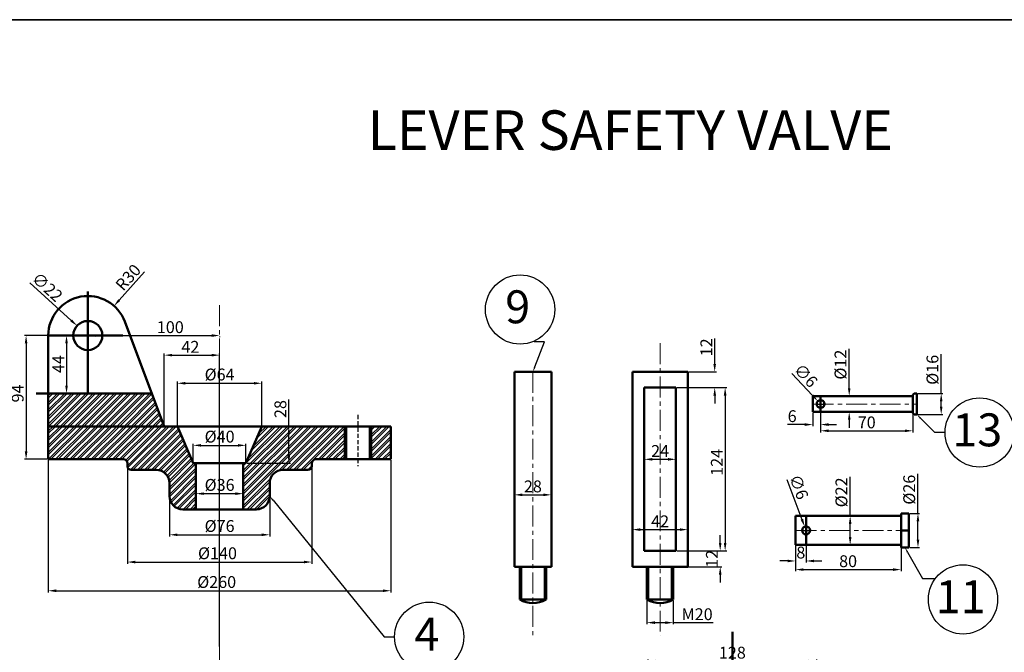
# Model space of a CAD drawing. Units: millimetres. Extents: x -282 to 2335, y -1129 to 664.
# Tile 6 of 8: x 594 to 1341, y 183 to 664. Entities that reach past the tile are written whole.
import ezdxf
from ezdxf import colors
from ezdxf.entities.mleader import LeaderData, LeaderLine
from ezdxf.math import Vec2, Vec3

# ---------------------------------------------------------------- set-up
doc = ezdxf.new("R2010")
doc.units = ezdxf.units.MM
doc.header["$LTSCALE"] = 0.5
doc.linetypes.add('CENTER', pattern=[50.8, 31.75, -6.35, 6.35, -6.35])
doc.linetypes.add('HIDDEN', pattern=[9.525, 6.35, -3.175])
for name, color, linetype, lineweight in [('M-CNTR', 1, 'CENTER', 18), ('M-DIMS', 2, 'Continuous', 25), ('M-HATC', 8, 'Continuous', 18), ('M-HIDN', 4, 'HIDDEN', 25), ('M-OUTL', 7, 'Continuous', 50), ('M-TEXT', 3, 'Continuous', 25), ('M-TTLB', 7, 'Continuous', 35)]:
    doc.layers.add(name, color=color, linetype=linetype, lineweight=lineweight)
doc.styles.get("Standard").update_dxf_attribs({"font": 'arial.ttf'})
doc.dimstyles.new('ISO-25', dxfattribs={"dimtxt": 9, "dimasz": 6, "dimexe": 1.25, "dimexo": 0.625, "dimtad": 1, "dimtxsty": 'Standard', "dimcen": 2.5, "dimadec": 0, "dimazin": 0, "dimtfac": 1, "dimtofl": 0, "dimtmove": 0, "dimatfit": 3, "dimfxl": 1, "dimarcsym": 0})

# ---------------------------------------------------------------- blocks, each defined once
blk = doc.blocks.new('*D30')
at = {"layer": 'Defpoints', "color": 0, "transparency": 16777216}
for p in [(645.29, 423.91), (629.15, 379.91), (645.29, 379.91)]:
    blk.add_point(p, dxfattribs=at)
at = {"layer": 'M-DIMS', "color": 0, "lineweight": -2, "transparency": 16777216}
for p, q in [((644.66, 423.91), (627.9, 423.91)), ((629.15, 417.91), (629.15, 385.91)), ((644.66, 379.91), (627.9, 379.91))]:
    blk.add_line(p, q, dxfattribs=at)
at = {"layer": 'M-DIMS', "color": 0, "transparency": 16777216}
for points in [[(628.15, 417.91), (630.15, 417.91), (629.15, 423.91)], [(628.15, 385.91), (630.15, 385.91), (629.15, 379.91)]]:
    blk.add_solid(points, dxfattribs=at)
at = {"layer": 'M-DIMS', "color": 0, "transparency": 16777216, "insert": (624.02, 402.22), "char_height": 9, "attachment_point": 5, "rotation": 90}
blk.add_mtext('44', dxfattribs=at)
blk = doc.blocks.new('*D31')
at = {"layer": 'Defpoints', "color": 0, "transparency": 16777216}
for p in [(645.29, 423.91), (598.46, 329.91), (615.29, 329.91)]:
    blk.add_point(p, dxfattribs=at)
at = {"layer": 'M-DIMS', "color": 0, "lineweight": -2, "transparency": 16777216}
for p, q in [((644.66, 423.91), (597.21, 423.91)), ((598.46, 417.91), (598.46, 335.91)), ((614.66, 329.91), (597.21, 329.91))]:
    blk.add_line(p, q, dxfattribs=at)
at = {"layer": 'M-DIMS', "color": 0, "transparency": 16777216}
for points in [[(597.46, 417.91), (599.46, 417.91), (598.46, 423.91)], [(597.46, 335.91), (599.46, 335.91), (598.46, 329.91)]]:
    blk.add_solid(points, dxfattribs=at)
at = {"layer": 'M-DIMS', "color": 0, "transparency": 16777216, "insert": (593.24, 379.91), "char_height": 9, "attachment_point": 5, "rotation": 90}
blk.add_mtext('94', dxfattribs=at)
blk = doc.blocks.new('*D32')
at = {"layer": 'Defpoints', "color": 0, "transparency": 16777216}
for p in [(645.29, 423.91), (745.29, 423.91), (745.29, 423.88)]:
    blk.add_point(p, dxfattribs=at)
at = {"layer": 'M-DIMS', "color": 0, "lineweight": -2, "transparency": 16777216}
for p, q in [((645.29, 423.29), (645.29, 422.63)), ((651.29, 423.88), (739.29, 423.88)), ((745.29, 423.29), (745.29, 422.63))]:
    blk.add_line(p, q, dxfattribs=at)
at = {"layer": 'M-DIMS', "color": 0, "transparency": 16777216}
for points in [[(651.29, 424.88), (651.29, 422.88), (645.29, 423.88)], [(739.29, 424.88), (739.29, 422.88), (745.29, 423.88)]]:
    blk.add_solid(points, dxfattribs=at)
at = {"layer": 'M-DIMS', "color": 0, "transparency": 16777216, "insert": (707.89, 429.1), "char_height": 9, "attachment_point": 5}
blk.add_mtext('100', dxfattribs=at)
blk = doc.blocks.new('*D33')
at = {"layer": 'Defpoints', "color": 0, "transparency": 16777216}
for p in [(745.29, 409), (703.29, 354.91), (745.29, 187.04)]:
    blk.add_point(p, dxfattribs=at)
at = {"layer": 'M-DIMS', "color": 0, "lineweight": -2, "transparency": 16777216}
for p, q in [((703.29, 355.54), (703.29, 410.25)), ((709.29, 409), (739.29, 409)), ((745.29, 187.66), (745.29, 410.25))]:
    blk.add_line(p, q, dxfattribs=at)
at = {"layer": 'M-DIMS', "color": 0, "transparency": 16777216}
for points in [[(709.29, 410), (709.29, 408), (703.29, 409)], [(739.29, 410), (739.29, 408), (745.29, 409)]]:
    blk.add_solid(points, dxfattribs=at)
at = {"layer": 'M-DIMS', "color": 0, "transparency": 16777216, "insert": (723.11, 414.14), "char_height": 9, "attachment_point": 5}
blk.add_mtext('42', dxfattribs=at)
blk = doc.blocks.new('*D34')
at = {"layer": 'Defpoints', "color": 0, "transparency": 16777216}
for p in [(777.29, 387.65), (713.29, 354.91), (777.29, 354.91)]:
    blk.add_point(p, dxfattribs=at)
at = {"layer": 'M-DIMS', "color": 0, "lineweight": -2, "transparency": 16777216}
for p, q in [((713.29, 355.54), (713.29, 388.9)), ((777.29, 355.54), (777.29, 388.9)), ((719.29, 387.65), (771.29, 387.65))]:
    blk.add_line(p, q, dxfattribs=at)
at = {"layer": 'M-DIMS', "color": 0, "transparency": 16777216}
for points in [[(719.29, 388.65), (719.29, 386.65), (713.29, 387.65)], [(771.29, 388.65), (771.29, 386.65), (777.29, 387.65)]]:
    blk.add_solid(points, dxfattribs=at)
at = {"layer": 'M-DIMS', "color": 0, "transparency": 16777216, "insert": (745.29, 393.13), "char_height": 9, "attachment_point": 5}
blk.add_mtext('%%C64', dxfattribs=at)
blk = doc.blocks.new('*D35')
at = {"layer": 'Defpoints', "color": 0, "transparency": 16777216}
for p in [(765.29, 340.5), (725.29, 326.91), (765.29, 326.91)]:
    blk.add_point(p, dxfattribs=at)
at = {"layer": 'M-DIMS', "color": 0, "lineweight": -2, "transparency": 16777216}
for p, q in [((725.29, 327.54), (725.29, 341.75)), ((731.29, 340.5), (759.29, 340.5)), ((765.29, 327.54), (765.29, 341.75))]:
    blk.add_line(p, q, dxfattribs=at)
at = {"layer": 'M-DIMS', "color": 0, "transparency": 16777216}
for points in [[(731.29, 341.5), (731.29, 339.5), (725.29, 340.5)], [(759.29, 341.5), (759.29, 339.5), (765.29, 340.5)]]:
    blk.add_solid(points, dxfattribs=at)
at = {"layer": 'M-DIMS', "color": 0, "transparency": 16777216, "insert": (745.29, 345.97), "char_height": 9, "attachment_point": 5}
blk.add_mtext('%%C40', dxfattribs=at)
blk = doc.blocks.new('*D36')
at = {"layer": 'Defpoints', "color": 0, "transparency": 16777216}
for p in [(727.29, 299.05), (763.29, 303.82), (763.29, 299.05)]:
    blk.add_point(p, dxfattribs=at)
at = {"layer": 'M-DIMS', "color": 0, "lineweight": -2, "transparency": 16777216}
for p, q in [((727.29, 299.68), (727.29, 305.07)), ((733.29, 303.82), (757.29, 303.82)), ((763.29, 299.68), (763.29, 305.07))]:
    blk.add_line(p, q, dxfattribs=at)
at = {"layer": 'M-DIMS', "color": 0, "transparency": 16777216}
for points in [[(733.29, 304.82), (733.29, 302.82), (727.29, 303.82)], [(757.29, 304.82), (757.29, 302.82), (763.29, 303.82)]]:
    blk.add_solid(points, dxfattribs=at)
at = {"layer": 'M-DIMS', "color": 0, "transparency": 16777216, "insert": (745.29, 309.29), "char_height": 9, "attachment_point": 5}
blk.add_mtext('%%C36', dxfattribs=at)
blk = doc.blocks.new('*D37')
at = {"layer": 'Defpoints', "color": 0, "transparency": 16777216}
for p in [(707.29, 306.91), (783.29, 306.91), (783.29, 272.6)]:
    blk.add_point(p, dxfattribs=at)
at = {"layer": 'M-DIMS', "color": 0, "lineweight": -2, "transparency": 16777216}
for p, q in [((707.29, 306.29), (707.29, 271.35)), ((783.29, 306.29), (783.29, 271.35)), ((713.29, 272.6), (777.29, 272.6))]:
    blk.add_line(p, q, dxfattribs=at)
at = {"layer": 'M-DIMS', "color": 0, "transparency": 16777216}
for points in [[(713.29, 273.6), (713.29, 271.6), (707.29, 272.6)], [(777.29, 273.6), (777.29, 271.6), (783.29, 272.6)]]:
    blk.add_solid(points, dxfattribs=at)
at = {"layer": 'M-DIMS', "color": 0, "transparency": 16777216, "insert": (745.29, 278.08), "char_height": 9, "attachment_point": 5}
blk.add_mtext('%%C76', dxfattribs=at)
blk = doc.blocks.new('*D38')
at = {"layer": 'Defpoints', "color": 0, "transparency": 16777216}
for p in [(675.29, 325.91), (815.29, 325.91), (815.29, 251.9)]:
    blk.add_point(p, dxfattribs=at)
at = {"layer": 'M-DIMS', "color": 0, "lineweight": -2, "transparency": 16777216}
for p, q in [((675.29, 325.29), (675.29, 250.65)), ((815.29, 325.29), (815.29, 250.65)), ((681.29, 251.9), (809.29, 251.9))]:
    blk.add_line(p, q, dxfattribs=at)
at = {"layer": 'M-DIMS', "color": 0, "transparency": 16777216}
for points in [[(681.29, 252.9), (681.29, 250.9), (675.29, 251.9)], [(809.29, 252.9), (809.29, 250.9), (815.29, 251.9)]]:
    blk.add_solid(points, dxfattribs=at)
at = {"layer": 'M-DIMS', "color": 0, "transparency": 16777216, "insert": (743.69, 257.38), "char_height": 9, "attachment_point": 5}
blk.add_mtext('%%C140', dxfattribs=at)
blk = doc.blocks.new('*D39')
at = {"layer": 'Defpoints', "color": 0, "transparency": 16777216}
for p in [(615.29, 329.91), (875.29, 329.91), (875.29, 230.09)]:
    blk.add_point(p, dxfattribs=at)
at = {"layer": 'M-DIMS', "color": 0, "lineweight": -2, "transparency": 16777216}
for p, q in [((615.29, 329.29), (615.29, 228.84)), ((875.29, 329.29), (875.29, 228.84)), ((621.29, 230.09), (869.29, 230.09))]:
    blk.add_line(p, q, dxfattribs=at)
at = {"layer": 'M-DIMS', "color": 0, "transparency": 16777216}
for points in [[(621.29, 231.09), (621.29, 229.09), (615.29, 230.09)], [(869.29, 231.09), (869.29, 229.09), (875.29, 230.09)]]:
    blk.add_solid(points, dxfattribs=at)
at = {"layer": 'M-DIMS', "color": 0, "transparency": 16777216, "insert": (743.06, 235.56), "char_height": 9, "attachment_point": 5}
blk.add_mtext('%%C260', dxfattribs=at)
blk = doc.blocks.new('*D40')
at = {"layer": 'Defpoints', "color": 0, "transparency": 16777216}
for p in [(637.14, 431.3), (653.43, 416.52)]:
    blk.add_point(p, dxfattribs=at)
at = {"layer": 'M-DIMS', "color": 0, "lineweight": -2, "transparency": 16777216}
for p, q in [((601.26, 463.84), (632.69, 435.33)), ((645.29, 421.41), (645.29, 426.41)), ((642.79, 423.91), (647.79, 423.91))]:
    blk.add_line(p, q, dxfattribs=at)
at = {"layer": 'M-DIMS', "color": 0, "transparency": 16777216}
blk.add_solid([(633.37, 436.07), (632.02, 434.59), (637.14, 431.3)], dxfattribs=at)
at = {"layer": 'M-DIMS', "color": 0, "transparency": 16777216, "insert": (613.76, 459.89), "char_height": 9, "attachment_point": 5, "rotation": 317.79433}
blk.add_mtext('∅22', dxfattribs=at)
blk = doc.blocks.new('*D41')
at = {"layer": 'Defpoints', "color": 0, "transparency": 16777216}
for p in [(665.18, 446.36), (645.29, 423.91)]:
    blk.add_point(p, dxfattribs=at)
at = {"layer": 'M-DIMS', "color": 0, "lineweight": -2, "transparency": 16777216}
for p, q in [((688.21, 472.35), (669.16, 450.86)), ((645.29, 421.41), (645.29, 426.41)), ((642.79, 423.91), (647.79, 423.91))]:
    blk.add_line(p, q, dxfattribs=at)
at = {"layer": 'M-DIMS', "color": 0, "transparency": 16777216}
blk.add_solid([(668.41, 451.52), (669.91, 450.19), (665.18, 446.36)], dxfattribs=at)
at = {"layer": 'M-DIMS', "color": 0, "transparency": 16777216, "insert": (676.77, 467.31), "char_height": 9, "attachment_point": 5, "rotation": 48.45504}
blk.add_mtext('R30', dxfattribs=at)
blk = doc.blocks.new('*D42')
at = {"layer": 'Defpoints', "color": 0, "transparency": 16777216}
for p in [(777.29, 354.91), (765.29, 326.91), (797.82, 326.91)]:
    blk.add_point(p, dxfattribs=at)
at = {"layer": 'M-DIMS', "color": 0, "lineweight": -2, "transparency": 16777216}
for p, q in [((797.82, 354.91), (797.82, 375.23)), ((777.91, 354.91), (799.07, 354.91)), ((797.82, 332.91), (797.82, 348.91)), ((765.91, 326.91), (799.07, 326.91))]:
    blk.add_line(p, q, dxfattribs=at)
at = {"layer": 'M-DIMS', "color": 0, "transparency": 16777216}
for points in [[(796.82, 348.91), (798.82, 348.91), (797.82, 354.91)], [(796.82, 332.91), (798.82, 332.91), (797.82, 326.91)]]:
    blk.add_solid(points, dxfattribs=at)
at = {"layer": 'M-DIMS', "color": 0, "transparency": 16777216, "insert": (792.6, 368.07), "char_height": 9, "attachment_point": 5, "rotation": 90}
blk.add_mtext('28', dxfattribs=at)
blk = doc.blocks.new('*D47')
at = {"layer": 'Defpoints', "color": 0, "transparency": 16777216}
for p in [(1100.55, 396.35), (1091.55, 384.35), (1120.98, 384.35)]:
    blk.add_point(p, dxfattribs=at)
at = {"layer": 'M-DIMS', "color": 0, "lineweight": -2, "transparency": 16777216}
for p, q in [((1120.98, 402.35), (1120.98, 421.55)), ((1101.17, 396.35), (1122.23, 396.35)), ((1092.17, 384.35), (1122.23, 384.35)), ((1120.98, 378.35), (1120.98, 372.35))]:
    blk.add_line(p, q, dxfattribs=at)
at = {"layer": 'M-DIMS', "color": 0, "transparency": 16777216}
for points in [[(1119.98, 402.35), (1121.98, 402.35), (1120.98, 396.35)], [(1119.98, 378.35), (1121.98, 378.35), (1120.98, 384.35)]]:
    blk.add_solid(points, dxfattribs=at)
at = {"layer": 'M-DIMS', "color": 0, "transparency": 16777216, "insert": (1115.84, 414.95), "char_height": 9, "attachment_point": 5, "rotation": 90}
blk.add_mtext('12', dxfattribs=at)
blk = doc.blocks.new('*D48')
at = {"layer": 'Defpoints', "color": 0, "transparency": 16777216}
for p in [(1067.55, 329.9), (1091.55, 329.9), (1091.55, 329.9)]:
    blk.add_point(p, dxfattribs=at)
at = {"layer": 'M-DIMS', "color": 0, "lineweight": -2, "transparency": 16777216}
for p, q in [((1067.55, 330.53), (1067.55, 331.15)), ((1073.55, 329.9), (1085.55, 329.9)), ((1091.55, 330.53), (1091.55, 331.15))]:
    blk.add_line(p, q, dxfattribs=at)
at = {"layer": 'M-DIMS', "color": 0, "transparency": 16777216}
for points in [[(1073.55, 330.9), (1073.55, 328.9), (1067.55, 329.9)], [(1085.55, 330.9), (1085.55, 328.9), (1091.55, 329.9)]]:
    blk.add_solid(points, dxfattribs=at)
at = {"layer": 'M-DIMS', "color": 0, "transparency": 16777216, "insert": (1079.55, 335.04), "char_height": 9, "attachment_point": 5}
blk.add_mtext('24', dxfattribs=at)
blk = doc.blocks.new('*D49')
at = {"layer": 'Defpoints', "color": 0, "transparency": 16777216}
for p in [(1100.55, 276.52), (1058.55, 271.29), (1100.55, 271.29)]:
    blk.add_point(p, dxfattribs=at)
at = {"layer": 'M-DIMS', "color": 0, "lineweight": -2, "transparency": 16777216}
for p, q in [((1058.55, 271.92), (1058.55, 277.77)), ((1064.55, 276.52), (1094.55, 276.52)), ((1100.55, 271.92), (1100.55, 277.77))]:
    blk.add_line(p, q, dxfattribs=at)
at = {"layer": 'M-DIMS', "color": 0, "transparency": 16777216}
for points in [[(1064.55, 277.52), (1064.55, 275.52), (1058.55, 276.52)], [(1094.55, 277.52), (1094.55, 275.52), (1100.55, 276.52)]]:
    blk.add_solid(points, dxfattribs=at)
at = {"layer": 'M-DIMS', "color": 0, "transparency": 16777216, "insert": (1079.55, 281.66), "char_height": 9, "attachment_point": 5}
blk.add_mtext('42', dxfattribs=at)
blk = doc.blocks.new('*D50')
at = {"layer": 'Defpoints', "color": 0, "transparency": 16777216}
for p in [(1120.98, 384.35), (1091.55, 260.35), (1128.9, 260.35)]:
    blk.add_point(p, dxfattribs=at)
at = {"layer": 'M-DIMS', "color": 0, "lineweight": -2, "transparency": 16777216}
for p, q in [((1121.61, 384.35), (1130.15, 384.35)), ((1128.9, 378.35), (1128.9, 266.35)), ((1092.17, 260.35), (1130.15, 260.35))]:
    blk.add_line(p, q, dxfattribs=at)
at = {"layer": 'M-DIMS', "color": 0, "transparency": 16777216}
for points in [[(1127.9, 378.35), (1129.9, 378.35), (1128.9, 384.35)], [(1127.9, 266.35), (1129.9, 266.35), (1128.9, 260.35)]]:
    blk.add_solid(points, dxfattribs=at)
at = {"layer": 'M-DIMS', "color": 0, "transparency": 16777216, "insert": (1123.76, 327.6), "char_height": 9, "attachment_point": 5, "rotation": 90}
blk.add_mtext('124', dxfattribs=at)
blk = doc.blocks.new('*D51')
at = {"layer": 'Defpoints', "color": 0, "transparency": 16777216}
for p in [(1091.55, 260.35), (1091.55, 248.35), (1125.15, 248.35)]:
    blk.add_point(p, dxfattribs=at)
at = {"layer": 'M-DIMS', "color": 0, "lineweight": -2, "transparency": 16777216}
for p, q in [((1125.15, 266.35), (1125.15, 272.35)), ((1092.17, 260.35), (1126.4, 260.35)), ((1092.17, 248.35), (1126.4, 248.35)), ((1125.15, 242.35), (1125.15, 236.35))]:
    blk.add_line(p, q, dxfattribs=at)
at = {"layer": 'M-DIMS', "color": 0, "transparency": 16777216}
for points in [[(1124.15, 266.35), (1126.15, 266.35), (1125.15, 260.35)], [(1124.15, 242.35), (1126.15, 242.35), (1125.15, 248.35)]]:
    blk.add_solid(points, dxfattribs=at)
at = {"layer": 'M-DIMS', "color": 0, "transparency": 16777216, "insert": (1120.01, 254.35), "char_height": 9, "attachment_point": 5, "rotation": 90}
blk.add_mtext('12', dxfattribs=at)
blk = doc.blocks.new('*D52')
at = {"layer": 'Defpoints', "color": 0, "transparency": 16777216}
for p in [(1069.55, 223.35), (1089.55, 223.35), (1089.55, 205.87)]:
    blk.add_point(p, dxfattribs=at)
at = {"layer": 'M-DIMS', "color": 0, "lineweight": -2, "transparency": 16777216}
for p, q in [((1069.55, 222.73), (1069.55, 204.62)), ((1089.55, 222.73), (1089.55, 204.62)), ((1075.55, 205.87), (1083.55, 205.87)), ((1089.55, 205.87), (1119.72, 205.87))]:
    blk.add_line(p, q, dxfattribs=at)
at = {"layer": 'M-DIMS', "color": 0, "transparency": 16777216}
for points in [[(1075.55, 206.87), (1075.55, 204.87), (1069.55, 205.87)], [(1083.55, 206.87), (1083.55, 204.87), (1089.55, 205.87)]]:
    blk.add_solid(points, dxfattribs=at)
at = {"layer": 'M-DIMS', "color": 0, "transparency": 16777216, "insert": (1107.64, 211.09), "char_height": 9, "attachment_point": 5}
blk.add_mtext('M20', dxfattribs=at)
blk = doc.blocks.new('*D53')
at = {"layer": 'Defpoints', "color": 0, "transparency": 16777216}
for p in [(969.02, 302.93), (997.02, 302.93), (997.02, 302.93)]:
    blk.add_point(p, dxfattribs=at)
at = {"layer": 'M-DIMS', "color": 0, "lineweight": -2, "transparency": 16777216}
for p, q in [((969.02, 303.56), (969.02, 304.18)), ((975.02, 302.93), (991.02, 302.93)), ((997.02, 303.56), (997.02, 304.18))]:
    blk.add_line(p, q, dxfattribs=at)
at = {"layer": 'M-DIMS', "color": 0, "transparency": 16777216}
for points in [[(975.02, 303.93), (975.02, 301.93), (969.02, 302.93)], [(991.02, 303.93), (991.02, 301.93), (997.02, 302.93)]]:
    blk.add_solid(points, dxfattribs=at)
at = {"layer": 'M-DIMS', "color": 0, "transparency": 16777216, "insert": (983.02, 308.15), "char_height": 9, "attachment_point": 5}
blk.add_mtext('28', dxfattribs=at)
blk = doc.blocks.new('*D62')
at = {"layer": 'Defpoints', "color": 0, "transparency": 16777216}
for p in [(1198.37, 176.66), (1070.37, 152.45), (1198.37, 152.45)]:
    blk.add_point(p, dxfattribs=at)
at = {"layer": 'M-DIMS', "color": 0, "lineweight": -2, "transparency": 16777216}
for p, q in [((1070.37, 153.08), (1070.37, 177.91)), ((1076.37, 176.66), (1192.37, 176.66)), ((1198.37, 153.08), (1198.37, 177.91))]:
    blk.add_line(p, q, dxfattribs=at)
at = {"layer": 'M-DIMS', "color": 0, "transparency": 16777216}
for points in [[(1076.37, 177.66), (1076.37, 175.66), (1070.37, 176.66)], [(1192.37, 177.66), (1192.37, 175.66), (1198.37, 176.66)]]:
    blk.add_solid(points, dxfattribs=at)
at = {"layer": 'M-DIMS', "color": 0, "transparency": 16777216, "insert": (1134.37, 181.88), "char_height": 9, "attachment_point": 5}
blk.add_mtext('128', dxfattribs=at)
blk = doc.blocks.new('*D72')
at = {"layer": 'Defpoints', "color": 0, "transparency": 16777216}
for p in [(1274.36, 379.9), (1274.36, 363.9), (1292.85, 363.9)]:
    blk.add_point(p, dxfattribs=at)
at = {"layer": 'M-DIMS', "color": 0, "lineweight": -2, "transparency": 16777216}
for p, q in [((1292.85, 379.9), (1292.85, 409.83)), ((1274.98, 379.9), (1294.1, 379.9)), ((1292.85, 369.9), (1292.85, 373.9)), ((1274.98, 363.9), (1294.1, 363.9))]:
    blk.add_line(p, q, dxfattribs=at)
at = {"layer": 'M-DIMS', "color": 0, "transparency": 16777216}
for points in [[(1291.85, 373.9), (1293.85, 373.9), (1292.85, 379.9)], [(1291.85, 369.9), (1293.85, 369.9), (1292.85, 363.9)]]:
    blk.add_solid(points, dxfattribs=at)
at = {"layer": 'M-DIMS', "color": 0, "transparency": 16777216, "insert": (1287.38, 397.87), "char_height": 9, "attachment_point": 5, "rotation": 90}
blk.add_mtext('%%C16', dxfattribs=at)
blk = doc.blocks.new('*D73')
at = {"layer": 'Defpoints', "color": 0, "transparency": 16777216}
for p in [(1195.36, 365.9), (1201.36, 365.9), (1201.36, 356.28)]:
    blk.add_point(p, dxfattribs=at)
at = {"layer": 'M-DIMS', "color": 0, "lineweight": -2, "transparency": 16777216}
for p, q in [((1195.36, 365.28), (1195.36, 355.03)), ((1201.36, 365.28), (1201.36, 355.03)), ((1189.36, 356.28), (1176.16, 356.28)), ((1207.36, 356.28), (1213.36, 356.28))]:
    blk.add_line(p, q, dxfattribs=at)
at = {"layer": 'M-DIMS', "color": 0, "transparency": 16777216}
for points in [[(1189.36, 357.28), (1189.36, 355.28), (1195.36, 356.28)], [(1207.36, 357.28), (1207.36, 355.28), (1201.36, 356.28)]]:
    blk.add_solid(points, dxfattribs=at)
at = {"layer": 'M-DIMS', "color": 0, "transparency": 16777216, "insert": (1179.76, 361.5), "char_height": 9, "attachment_point": 5}
blk.add_mtext('6', dxfattribs=at)
blk = doc.blocks.new('*D74')
at = {"layer": 'Defpoints', "color": 0, "transparency": 16777216}
for p in [(1201.36, 365.9), (1271.36, 365.9), (1271.36, 351.56)]:
    blk.add_point(p, dxfattribs=at)
at = {"layer": 'M-DIMS', "color": 0, "lineweight": -2, "transparency": 16777216}
for p, q in [((1201.36, 365.28), (1201.36, 350.31)), ((1271.36, 365.28), (1271.36, 350.31)), ((1207.36, 351.56), (1265.36, 351.56))]:
    blk.add_line(p, q, dxfattribs=at)
at = {"layer": 'M-DIMS', "color": 0, "transparency": 16777216}
for points in [[(1207.36, 352.56), (1207.36, 350.56), (1201.36, 351.56)], [(1265.36, 352.56), (1265.36, 350.56), (1271.36, 351.56)]]:
    blk.add_solid(points, dxfattribs=at)
at = {"layer": 'M-DIMS', "color": 0, "transparency": 16777216, "insert": (1236.33, 356.78), "char_height": 9, "attachment_point": 5}
blk.add_mtext('70', dxfattribs=at)
blk = doc.blocks.new('*D75')
at = {"layer": 'Defpoints', "color": 0, "transparency": 16777216}
for p in [(1223.05, 377.9), (1228.96, 377.9), (1228.96, 365.9)]:
    blk.add_point(p, dxfattribs=at)
at = {"layer": 'M-DIMS', "color": 0, "lineweight": -2, "transparency": 16777216}
for p, q in [((1223.05, 383.9), (1223.05, 413.75)), ((1228.34, 377.9), (1221.8, 377.9)), ((1228.34, 365.9), (1221.8, 365.9)), ((1223.05, 359.9), (1223.05, 353.9))]:
    blk.add_line(p, q, dxfattribs=at)
at = {"layer": 'M-DIMS', "color": 0, "transparency": 16777216}
for points in [[(1222.05, 383.9), (1224.05, 383.9), (1223.05, 377.9)], [(1222.05, 359.9), (1224.05, 359.9), (1223.05, 365.9)]]:
    blk.add_solid(points, dxfattribs=at)
at = {"layer": 'M-DIMS', "color": 0, "transparency": 16777216, "insert": (1217.58, 401.82), "char_height": 9, "attachment_point": 5, "rotation": 90}
blk.add_mtext('%%C12', dxfattribs=at)
blk = doc.blocks.new('*D76')
at = {"layer": 'Defpoints', "color": 0, "transparency": 16777216}
for p in [(1199.3, 374.09), (1203.41, 369.72)]:
    blk.add_point(p, dxfattribs=at)
at = {"layer": 'M-DIMS', "color": 0, "lineweight": -2, "transparency": 16777216}
for p, q in [((1179.45, 395.14), (1195.18, 378.45)), ((1201.36, 369.4), (1201.36, 374.4)), ((1198.86, 371.9), (1203.86, 371.9))]:
    blk.add_line(p, q, dxfattribs=at)
at = {"layer": 'M-DIMS', "color": 0, "transparency": 16777216}
blk.add_solid([(1195.91, 379.14), (1194.45, 377.77), (1199.3, 374.09)], dxfattribs=at)
at = {"layer": 'M-DIMS', "color": 0, "transparency": 16777216, "insert": (1189.24, 392.73), "char_height": 9, "attachment_point": 5, "rotation": 313.30697}
blk.add_mtext('∅6', dxfattribs=at)
blk = doc.blocks.new('*D77')
at = {"layer": 'Defpoints', "color": 0, "transparency": 16777216}
for p in [(1189.27, 278.68), (1191.42, 273.08)]:
    blk.add_point(p, dxfattribs=at)
at = {"layer": 'M-DIMS', "color": 0, "lineweight": -2, "transparency": 16777216}
for p, q in [((1175.59, 314.49), (1187.13, 284.29)), ((1190.34, 273.38), (1190.34, 278.38)), ((1187.84, 275.88), (1192.84, 275.88))]:
    blk.add_line(p, q, dxfattribs=at)
at = {"layer": 'M-DIMS', "color": 0, "transparency": 16777216}
blk.add_solid([(1188.07, 284.65), (1186.2, 283.93), (1189.27, 278.68)], dxfattribs=at)
at = {"layer": 'M-DIMS', "color": 0, "transparency": 16777216, "insert": (1183.72, 308.53), "char_height": 9, "attachment_point": 5, "rotation": 290.91824}
blk.add_mtext('∅6', dxfattribs=at)
blk = doc.blocks.new('*D78')
at = {"layer": 'Defpoints', "color": 0, "transparency": 16777216}
for p in [(1182.34, 275.88), (1190.34, 275.88), (1190.34, 252.71)]:
    blk.add_point(p, dxfattribs=at)
at = {"layer": 'M-DIMS', "color": 0, "lineweight": -2, "transparency": 16777216}
for p, q in [((1182.34, 275.26), (1182.34, 251.46)), ((1190.34, 275.26), (1190.34, 251.46)), ((1176.34, 252.71), (1170.34, 252.71)), ((1196.34, 252.71), (1202.34, 252.71))]:
    blk.add_line(p, q, dxfattribs=at)
at = {"layer": 'M-DIMS', "color": 0, "transparency": 16777216}
for points in [[(1176.34, 253.71), (1176.34, 251.71), (1182.34, 252.71)], [(1196.34, 253.71), (1196.34, 251.71), (1190.34, 252.71)]]:
    blk.add_solid(points, dxfattribs=at)
at = {"layer": 'M-DIMS', "color": 0, "transparency": 16777216, "insert": (1186.34, 257.93), "char_height": 9, "attachment_point": 5}
blk.add_mtext('8', dxfattribs=at)
blk = doc.blocks.new('*D79')
at = {"layer": 'Defpoints', "color": 0, "transparency": 16777216}
for p in [(1182.34, 264.88), (1262.34, 264.88), (1262.34, 246.14)]:
    blk.add_point(p, dxfattribs=at)
at = {"layer": 'M-DIMS', "color": 0, "lineweight": -2, "transparency": 16777216}
for p, q in [((1182.34, 264.26), (1182.34, 244.89)), ((1262.34, 264.26), (1262.34, 244.89)), ((1188.34, 246.14), (1256.34, 246.14))]:
    blk.add_line(p, q, dxfattribs=at)
at = {"layer": 'M-DIMS', "color": 0, "transparency": 16777216}
for points in [[(1188.34, 247.14), (1188.34, 245.14), (1182.34, 246.14)], [(1256.34, 247.14), (1256.34, 245.14), (1262.34, 246.14)]]:
    blk.add_solid(points, dxfattribs=at)
at = {"layer": 'M-DIMS', "color": 0, "transparency": 16777216, "insert": (1222.19, 251.36), "char_height": 9, "attachment_point": 5}
blk.add_mtext('80', dxfattribs=at)
blk = doc.blocks.new('*D80')
at = {"layer": 'Defpoints', "color": 0, "transparency": 16777216}
for p in [(1232.66, 286.88), (1223.76, 264.88), (1232.66, 264.88)]:
    blk.add_point(p, dxfattribs=at)
at = {"layer": 'M-DIMS', "color": 0, "lineweight": -2, "transparency": 16777216}
for p, q in [((1223.76, 286.88), (1223.76, 316.72)), ((1232.03, 286.88), (1222.51, 286.88)), ((1223.76, 270.88), (1223.76, 280.88)), ((1232.03, 264.88), (1222.51, 264.88))]:
    blk.add_line(p, q, dxfattribs=at)
at = {"layer": 'M-DIMS', "color": 0, "transparency": 16777216}
for points in [[(1222.76, 280.88), (1224.76, 280.88), (1223.76, 286.88)], [(1222.76, 270.88), (1224.76, 270.88), (1223.76, 264.88)]]:
    blk.add_solid(points, dxfattribs=at)
at = {"layer": 'M-DIMS', "color": 0, "transparency": 16777216, "insert": (1218.29, 304.8), "char_height": 9, "attachment_point": 5, "rotation": 90}
blk.add_mtext('%%C22', dxfattribs=at)
blk = doc.blocks.new('*D81')
at = {"layer": 'Defpoints', "color": 0, "transparency": 16777216}
for p in [(1268.34, 288.88), (1268.34, 262.88), (1275.21, 262.88)]:
    blk.add_point(p, dxfattribs=at)
at = {"layer": 'M-DIMS', "color": 0, "lineweight": -2, "transparency": 16777216}
for p, q in [((1275.21, 288.88), (1275.21, 318.81)), ((1268.97, 288.88), (1276.46, 288.88)), ((1275.21, 268.88), (1275.21, 282.88)), ((1268.97, 262.88), (1276.46, 262.88))]:
    blk.add_line(p, q, dxfattribs=at)
at = {"layer": 'M-DIMS', "color": 0, "transparency": 16777216}
for points in [[(1274.21, 282.88), (1276.21, 282.88), (1275.21, 288.88)], [(1274.21, 268.88), (1276.21, 268.88), (1275.21, 262.88)]]:
    blk.add_solid(points, dxfattribs=at)
at = {"layer": 'M-DIMS', "color": 0, "transparency": 16777216, "insert": (1269.74, 306.85), "char_height": 9, "attachment_point": 5, "rotation": 90}
blk.add_mtext('%%C26', dxfattribs=at)

msp = doc.modelspace()

# ---------------------------------------------------------------- hatches: boundary and pattern name
at = {"layer": 'M-HATC'}
h = msp.add_hatch(dxfattribs=at)
h.set_pattern_fill('ANSI32', color=256, scale=0.4)
h.paths.add_polyline_path([(693.885, 379.912), (645.287, 379.912), (615.287, 379.912), (615.287, 354.912), (703.287, 354.912)])
h = msp.add_hatch(dxfattribs=at)
h.set_pattern_fill('ANSI32', color=256, scale=0.4)
h.paths.add_polyline_path([(713.287, 354.912), (615.287, 354.912), (615.287, 329.912), (672.287, 329.912, -0.4142136), (675.287, 326.912), (675.287, 324.912, 0.4142136), (678.287, 321.912), (697.287, 321.912, -0.4142136), (707.287, 311.912), (707.287, 301.912, 0.4142136), (717.287, 291.912), (727.287, 291.912), (727.287, 326.912), (725.287, 326.912)])
h.paths.add_polyline_path([(840.287, 354.912), (777.287, 354.912), (765.287, 326.912), (763.287, 326.912), (763.287, 291.912), (773.287, 291.912, 0.4142136), (783.287, 301.912), (783.287, 311.912, -0.4142136), (793.287, 321.912), (812.287, 321.912, 0.4142136), (815.287, 324.912), (815.287, 326.912, -0.4142136), (818.287, 329.912), (840.287, 329.912)])
h.paths.add_polyline_path([(875.287, 354.912), (860.287, 354.912), (860.287, 329.912), (875.287, 329.912)])

# ---------------------------------------------------------------- linework, layer by layer
at = {"layer": 'M-CNTR'}
for p, q in [((745.287, 446.981), (745.287, -130.826)), ((1079.549, 418.16), (1079.549, 195.877)), ((983.019, 396.35), (983.019, 195.877)), ((1195.356, 371.904), (1274.356, 371.904)), ((1182.345, 275.882), (1262.345, 275.882))]:
    msp.add_line(p, q, dxfattribs=at)
at = {"layer": 'M-HIDN'}
msp.add_line((850.287, 363.595), (850.287, 324.586), dxfattribs=at)
at = {"layer": 'M-OUTL'}
for p, q in [((645.287, 411.532), (645.287, 457.373)), ((703.287, 354.912), (673.367, 434.472)), ((615.287, 329.912), (615.287, 423.912)), ((615.287, 423.912), (671.949, 423.912)), ((645.287, 423.912), (645.287, 379.912)), ((997.019, 396.35), (969.019, 396.35)), ((969.019, 248.35), (969.019, 396.35)), ((997.019, 248.35), (997.019, 396.35)), ((1058.549, 396.35), (1058.549, 248.35)), ((1100.549, 396.35), (1058.549, 396.35)), ((1100.549, 248.35), (1100.549, 396.35)), ((1091.549, 384.35), (1067.549, 384.35)), ((1067.549, 384.35), (1067.549, 260.35)), ((1091.549, 384.35), (1091.549, 260.35)), ((645.287, 379.912), (606.02, 379.912)), ((606.02, 379.912), (615.287, 379.912)), ((645.287, 379.912), (693.885, 379.912)), ((1195.356, 377.904), (1195.356, 365.904)), ((1271.356, 377.904), (1195.356, 377.904)), ((1201.356, 377.904), (1201.356, 365.904)), ((1272.356, 379.904), (1271.356, 378.904)), ((1271.356, 377.904), (1271.356, 378.904)), ((1271.356, 365.904), (1271.356, 377.904)), ((1272.356, 379.904), (1274.356, 379.904)), ((1274.356, 379.904), (1273.356, 379.904)), ((1274.356, 379.904), (1274.356, 363.904)), ((1195.356, 365.904), (1271.356, 365.904)), ((1271.356, 364.904), (1271.356, 365.904)), ((1272.356, 363.904), (1271.356, 364.904)), ((1274.356, 363.904), (1272.356, 363.904)), ((875.287, 354.912), (615.287, 354.912)), ((615.287, 354.912), (615.287, 329.912)), ((713.287, 354.912), (725.287, 326.912)), ((777.287, 354.912), (765.287, 326.912)), ((840.287, 354.912), (840.287, 329.912)), ((841.287, 354.912), (841.287, 329.912)), ((859.287, 354.912), (859.287, 329.912)), ((860.287, 354.912), (860.287, 329.912)), ((875.287, 329.912), (875.287, 354.912)), ((615.287, 329.912), (672.287, 329.912)), ((818.287, 329.912), (875.287, 329.912)), ((675.287, 326.912), (675.287, 324.912)), ((678.287, 321.912), (697.287, 321.912)), ((725.287, 326.912), (765.287, 326.912)), ((727.287, 326.912), (727.287, 291.912)), ((763.287, 326.912), (763.287, 291.912)), ((793.287, 321.912), (812.287, 321.912)), ((815.287, 326.912), (815.287, 324.912)), ((707.287, 311.912), (707.287, 301.912)), ((783.287, 311.912), (783.287, 301.912)), ((717.287, 291.912), (773.287, 291.912)), ((1182.345, 286.882), (1182.345, 264.882)), ((1262.345, 286.882), (1182.345, 286.882)), ((1190.345, 286.882), (1190.345, 264.882)), ((1268.345, 288.882), (1262.345, 288.882)), ((1262.345, 288.882), (1262.345, 286.882)), ((1262.345, 264.882), (1262.345, 286.882)), ((1268.345, 262.882), (1268.345, 288.882)), ((1262.345, 275.882), (1268.345, 275.882)), ((1182.345, 264.882), (1262.345, 264.882)), ((1262.345, 262.882), (1262.345, 264.882)), ((1268.345, 262.882), (1262.345, 262.882)), ((1067.549, 260.35), (1091.549, 260.35)), ((969.019, 248.35), (997.019, 248.35)), ((973.019, 223.35), (973.019, 248.35)), ((974.019, 223.35), (974.019, 248.35)), ((992.019, 223.35), (992.019, 248.35)), ((993.019, 223.35), (993.019, 248.35)), ((1058.549, 248.35), (1100.549, 248.35)), ((1069.549, 223.35), (1069.549, 248.35)), ((1070.549, 223.35), (1070.549, 248.35)), ((1088.549, 223.35), (1088.549, 248.35)), ((1089.549, 223.35), (1089.549, 248.35)), ((973.019, 223.35), (993.019, 223.35)), ((1069.549, 223.35), (1089.549, 223.35)), ((1134.367, 154.454), (1134.367, 198.875))]:
    msp.add_line(p, q, dxfattribs=at)
for centre, radius in [((645.287, 423.912), 11), ((1201.356, 371.904), 3), ((1190.345, 275.882), 3)]:
    msp.add_circle(centre, radius, dxfattribs=at)
for centre, radius, start, end in [((645.287, 423.912), 30, 20.609693, 180), ((672.287, 326.912), 3, 0, 90), ((818.287, 326.912), 3, 90, 180), ((678.287, 324.912), 3, 180, 270), ((697.287, 311.912), 10, 0, 90), ((793.287, 311.912), 10, 90, 180), ((812.287, 324.912), 3, 270, 0), ((717.287, 301.912), 10, 180, 270), ((773.287, 301.912), 10, 270, 0), ((983.019, 240.671), 20, 240, 300), ((1079.549, 240.671), 20, 240, 300)]:
    msp.add_arc(centre, radius, start, end, dxfattribs=at)
at = {"layer": 'M-TEXT'}
for centre in [(973.305, 443.672), (1322.035, 350.242), (1309.386, 223.5), (904.33, 195.171)]:
    msp.add_circle(centre, 26.287, dxfattribs=at)
at = {"layer": 'M-TTLB', "ltscale": 0.5}
msp.add_lwpolyline([(-281.776, 663.767), (2334.915, 663.767), (2334.915, -1128.523), (-281.776, -1128.523)], close=True, dxfattribs=at)

# ---------------------------------------------------------------- texts
at = {"layer": 'M-TEXT', "ltscale": 0.5, "insert": (857.48, 594.875), "char_height": 30, "attachment_point": 1}
msp.add_mtext_dynamic_manual_height_columns('LEVER SAFETY VALVE', width=490.87341, gutter_width=12.5, heights=[0], dxfattribs=at)
at = {"layer": 'M-TEXT', "char_height": 25, "attachment_point": 1}
for s, insert in [('\\pxqc;9', (958.972, 458.212)), ('\\pxqc;13', (1307.702, 364.782)), ('\\pxqc;11', (1295.053, 238.04)), ('\\pxqc;4', (889.997, 209.711))]:
    msp.add_mtext_dynamic_manual_height_columns(s, width=25, gutter_width=12.5, heights=[7.196], dxfattribs=dict(at, insert=insert))

# ---------------------------------------------------------------- dimensions: what is measured, and where the dimension line sits
at = {"layer": 'M-DIMS'}
dim = msp.add_radius_dim(center=(645.287, 423.912), mpoint=(665.183, 446.365), dimstyle='ISO-25', override={"dimclrd": 0, "dimclre": 0, "dimclrt": 0}, dxfattribs=at)
dim.commit()
dim.dimension.update_dxf_attribs({"geometry": '*D41', "text_midpoint": (676.768, 467.314)})
for p1, p2, picture, middle in [((653.435, 416.522), (637.139, 431.302), '*D40', (610.088, 455.834)), ((1191.416, 273.079), (1189.274, 278.684), '*D77', (1178.612, 306.577))]:
    dim = msp.add_diameter_dim_2p(p1=p1, p2=p2, dimstyle='ISO-25', override={"dimclrd": 0, "dimclre": 0, "dimclrt": 0}, dxfattribs=at)
    dim.commit()
    dim.dimension.update_dxf_attribs({"geometry": picture, "text_midpoint": middle, "dimtype": 163})
for base, p1, p2, picture, middle in [((745.287, 423.878), (645.287, 423.912), (745.287, 423.912), '*D32', (707.891, 423.878)), ((745.287, 408.997), (703.287, 354.912), (745.287, 187.037), '*D33', (723.113, 408.997)), ((1201.356, 356.277), (1195.356, 365.904), (1201.356, 365.904), '*D73', (1179.759, 356.277)), ((1271.356, 351.561), (1201.356, 365.904), (1271.356, 365.904), '*D74', (1236.325, 351.561)), ((1091.549, 329.901), (1067.549, 329.901), (1091.549, 329.901), '*D48', (1079.549, 329.901)), ((997.019, 302.933), (969.019, 302.933), (997.019, 302.933), '*D53', (983.019, 302.933)), ((1100.549, 276.521), (1058.549, 271.292), (1100.549, 271.292), '*D49', (1079.549, 276.521)), ((1190.345, 252.706), (1182.345, 275.882), (1190.345, 275.882), '*D78', (1186.345, 252.706)), ((1262.345, 246.14), (1182.345, 264.882), (1262.345, 264.882), '*D79', (1222.187, 246.14)), ((1198.367, 176.664), (1070.367, 152.454), (1198.367, 152.454), '*D62', (1134.367, 176.664))]:
    dim = msp.add_linear_dim(base=base, p1=p1, p2=p2, dimstyle='ISO-25', override={"dimclrd": 0, "dimclre": 0, "dimclrt": 0}, dxfattribs=at)
    dim.commit()
    dim.dimension.update_dxf_attribs({"geometry": picture, "text_midpoint": middle, "dimtype": 160})
for base, p1, p2, picture, middle in [((598.463, 329.912), (645.287, 423.912), (615.287, 329.912), '*D31', (598.463, 379.912)), ((629.149, 379.912), (645.287, 423.912), (645.287, 379.912), '*D30', (629.149, 402.223)), ((1120.983, 384.35), (1100.549, 396.35), (1091.549, 384.35), '*D47', (1120.983, 414.952)), ((1128.903, 260.35), (1120.983, 384.35), (1091.549, 260.35), '*D50', (1128.903, 327.597)), ((797.817, 326.912), (777.287, 354.912), (765.287, 326.912), '*D42', (797.817, 368.069)), ((1125.153, 248.35), (1091.549, 260.35), (1091.549, 248.35), '*D51', (1125.153, 254.35))]:
    dim = msp.add_linear_dim(base=base, p1=p1, p2=p2, angle=90, dimstyle='ISO-25', override={"dimclrd": 0, "dimclre": 0, "dimclrt": 0}, dxfattribs=at)
    dim.commit()
    dim.dimension.update_dxf_attribs({"geometry": picture, "text_midpoint": middle, "dimtype": 160})
for base, p1, p2, picture, middle in [((1223.055, 377.904), (1228.961, 365.904), (1228.961, 377.904), '*D75', (1223.055, 401.825)), ((1292.853, 363.904), (1274.356, 379.904), (1274.356, 363.904), '*D72', (1292.853, 397.868)), ((1223.761, 264.882), (1232.659, 286.882), (1232.659, 264.882), '*D80', (1223.761, 304.803)), ((1275.21, 262.882), (1268.345, 288.882), (1268.345, 262.882), '*D81', (1275.21, 306.846))]:
    dim = msp.add_linear_dim(base=base, p1=p1, p2=p2, angle=90, text='%%C<>', dimstyle='ISO-25', override={"dimclrd": 0, "dimclre": 0, "dimclrt": 0}, dxfattribs=at)
    dim.commit()
    dim.dimension.update_dxf_attribs({"geometry": picture, "text_midpoint": middle, "dimtype": 160})
dim = msp.add_diameter_dim_2p(p1=(1203.413, 369.721), p2=(1199.298, 374.087), dimstyle='ISO-25', override={"dimclrd": 0, "dimclre": 0, "dimclrt": 0}, dxfattribs=at)
dim.commit()
dim.dimension.update_dxf_attribs({"geometry": '*D76', "text_midpoint": (1189.241, 392.734)})
for base, p1, p2, text, picture, middle in [((777.287, 387.654), (713.287, 354.912), (777.287, 354.912), '%%C<>', '*D34', (745.287, 387.654)), ((765.287, 340.497), (725.287, 326.912), (765.287, 326.912), '%%C<>', '*D35', (745.287, 340.497)), ((875.287, 230.091), (615.287, 329.912), (875.287, 329.912), '%%C<>', '*D39', (743.057, 230.091)), ((815.287, 251.905), (675.287, 325.912), (815.287, 325.912), '%%C<>', '*D38', (743.69, 251.905)), ((763.287, 303.82), (727.287, 299.054), (763.287, 299.054), '%%C<>', '*D36', (745.287, 303.82)), ((783.287, 272.604), (707.287, 306.912), (783.287, 306.912), '%%C<>', '*D37', (745.287, 272.604)), ((1089.549, 205.867), (1069.549, 223.35), (1089.549, 223.35), 'M<>', '*D52', (1107.636, 205.867))]:
    dim = msp.add_linear_dim(base=base, p1=p1, p2=p2, text=text, dimstyle='ISO-25', override={"dimclrd": 0, "dimclre": 0, "dimclrt": 0}, dxfattribs=at)
    dim.commit()
    dim.dimension.update_dxf_attribs({"geometry": picture, "text_midpoint": middle, "dimtype": 160})

# ---------------------------------------------------------------- leaders
at = {"layer": 'M-TEXT', "ltscale": 0.5}
ml = msp.add_multileader_mtext('Standard', dxfattribs=at)
ml.set_content('', color=256)
ml.set_leader_properties()
ml.build(insert=Vec2(0, 0))
ctx = ml.context
ctx.base_point, ctx.plane_origin = Vec3(979.934, 419.225), Vec3(983.019, 396.35)
ctx.text_align_type = 2
notes = []
notes.append((ctx, [(1, (1, 1, 0), (991.934, 419.225), (-1, 0), 8, [(0, [(983.019, 396.35)], 0, [])])]))
ctx.mtext.insert, ctx.mtext.alignment, ctx.mtext.flow_direction = Vec3(981.934, 421.225), 3, 5
ml = msp.add_multileader_mtext('Standard', dxfattribs=at)
ml.set_content('', color=256)
ml.set_leader_properties()
ml.build(insert=Vec2(0, 0))
ctx = ml.context
ctx.base_point, ctx.plane_origin = Vec3(1295.75, 350.51), Vec3(1274.356, 363.904)
notes.append((ctx, [(0, (1, 1, 0), (1287.75, 350.51), (1, 0), 8, [(0, [(1274.356, 363.904)], 0, [])])]))
ctx.mtext.insert, ctx.mtext.flow_direction = Vec3(1297.75, 352.51), 5
ml = msp.add_multileader_mtext('Standard', dxfattribs=at)
ml.set_content('', color=256)
ml.set_leader_properties()
ml.build(insert=Vec2(0, 0))
ctx = ml.context
ctx.base_point, ctx.plane_origin = Vec3(878.043, 195.171), Vec3(783.287, 301.912)
notes.append((ctx, [(0, (1, 1, 0), (870.043, 195.171), (1, 0), 8, [(0, [(783.287, 301.912)], 0, [])])]))
ctx.mtext.insert, ctx.mtext.flow_direction = Vec3(880.043, 197.171), 5
ml = msp.add_multileader_mtext('Standard', dxfattribs=at)
ml.set_content('', color=256)
ml.set_leader_properties()
ml.build(insert=Vec2(0, 0))
ctx = ml.context
ctx.base_point, ctx.plane_origin = Vec3(1288.468, 239.419), Vec3(1265.345, 262.882)
notes.append((ctx, [(0, (1, 1, 0), (1278.745, 239.419), (1, 0), 9.723, [(0, [(1265.345, 262.882)], 0, [])])]))
ctx.mtext.insert, ctx.mtext.flow_direction = Vec3(1290.468, 241.419), 5
for ctx, leaders in notes:
    for number, flags, end, landing, length, lines in leaders:
        leader = LeaderData()
        leader.index, (leader.has_last_leader_line, leader.has_dogleg_vector, leader.attachment_direction) = number, flags
        leader.last_leader_point, leader.dogleg_vector, leader.dogleg_length = Vec3(end), Vec3(landing), length
        for number, points, colour, breaks in lines:
            line = LeaderLine()
            line.index, line.vertices, line.color, line.breaks = number, Vec3.list(points), colors.encode_raw_color(colour), breaks
            leader.lines.append(line)
        ctx.leaders.append(leader)

doc.saveas('drawing.dxf')
